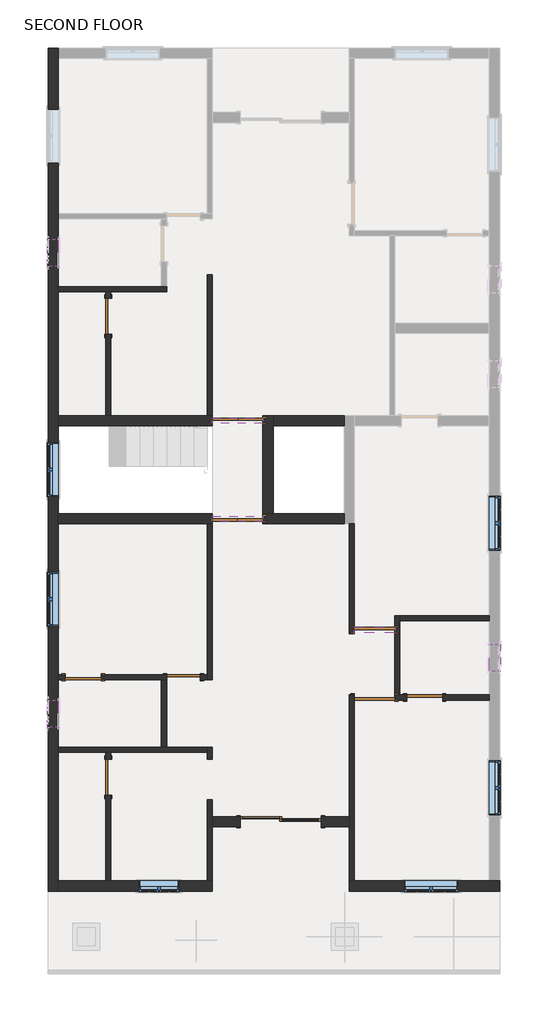
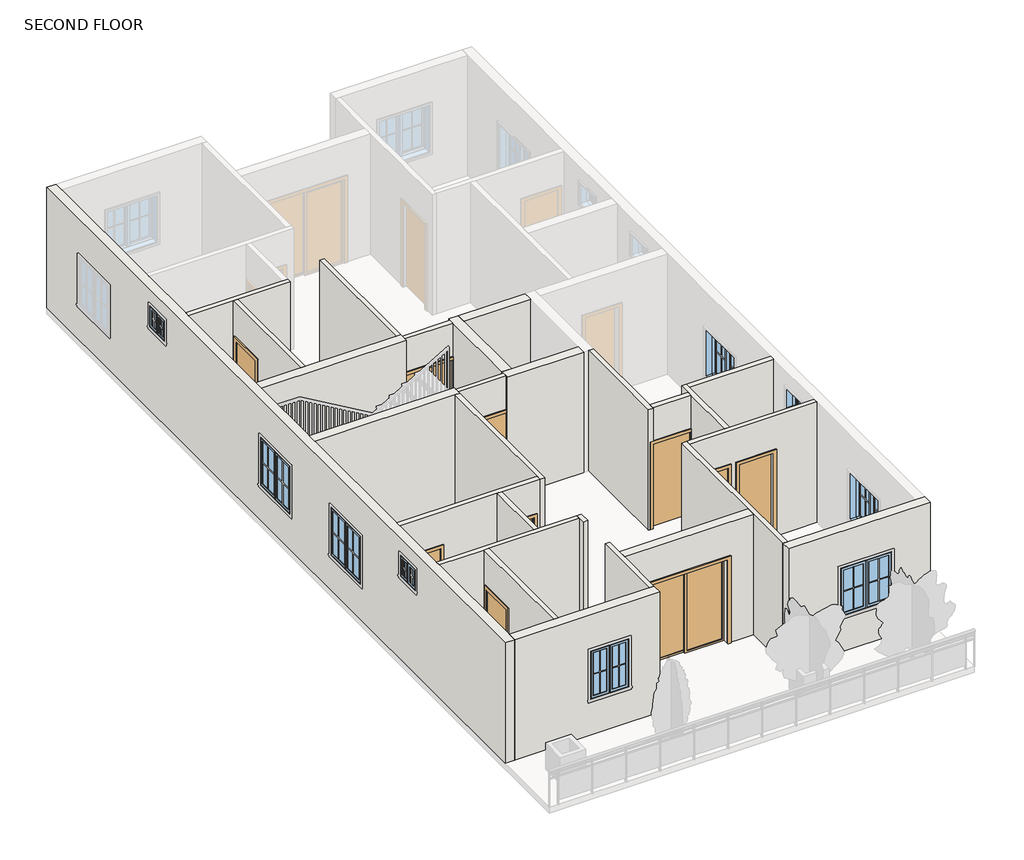
# One storey, part 1 of 4: 27 walls, 10 doors, 9 windows.
"""IFC4 building model written with IfcOpenShell, lengths in millimetres."""

from ifc_helpers import new_model, si_unit, frame, origin, place, context, project, spatial, polyline, outline, extrude, faceted_brep, transform, mapped, element, save
from components import door_31bd1cdd, door_d4d75d1e, door_214872d5, door_d141acb4, door_38851409, single_flush_3_x7_e5f9f3c4, single_flush_3_x7_305aa2a5, window_79894727, window_casement_double_3_x4_d341e8ac, window_casement_double_4_x4_af3140d2

model = new_model("IFC4")

# Units and contexts
model_context = context("Model", 3, world=origin())
ifc_project = project(units=[si_unit("LENGTHUNIT", "METRE", prefix="MILLI")], contexts=[model_context])

# Site, building, storey
site = spatial("IfcSite", under=ifc_project)
building = spatial("IfcBuilding", under=site)
storey = spatial("IfcBuildingStorey", under=building, Name="SECOND FLOOR", Elevation=6400.8)

# Doors
placement = place(None, origin())
door_shape = door_31bd1cdd(model_context)
element("IfcDoor", 1, ObjectType="Door-Double-Flush_Panel : 3'9\"X7'", at=placement, inside=storey, context=model_context, shape_type="MappedRepresentation", body=[
    mapped(door_shape, transform((-2091.0289041, 1664.1153263, 6400.8), x_axis=(1.0, 0.0, 0.0), y_axis=(0.0, 1.0, 0.0), z_axis=(0.0, 0.0, 1.0))),
])
element("IfcDoor", 2, ObjectType="Door-Double-Flush_Panel : 3'9\"X7'", at=placement, inside=storey, context=model_context, shape_type="MappedRepresentation", body=[
    mapped(door_shape, transform((-2091.0289041, -545.7007836, 6400.8), x_axis=(-1.0, 0.0, 0.0), y_axis=(0.0, -1.0, 0.0), z_axis=(0.0, 0.0, 1.0))),
])
door_2_shape = door_d4d75d1e(model_context)
element("IfcDoor", 3, ObjectType="Door-Double-Sliding : 72\" x 84\"", at=placement, inside=storey, context=model_context, shape_type="MappedRepresentation", body=[
    mapped(door_2_shape, transform((-1119.4789041, -7505.2846737, 6400.8), x_axis=(1.0, 0.0, 0.0), y_axis=(0.0, 1.0, 0.0), z_axis=(0.0, 0.0, 1.0))),
])
door_3_shape = door_214872d5(model_context)
element("IfcDoor", 4, ObjectType="Single-Flush : 2'6\"X7'", at=placement, inside=storey, context=model_context, shape_type="MappedRepresentation", body=[
    mapped(door_3_shape, transform((-3310.2289041, -4120.7346737, 6400.8), x_axis=(1.0, 0.0, 0.0), y_axis=(0.0, 1.0, 0.0), z_axis=(0.0, 0.0, 1.0))),
])
door_4_shape = door_d141acb4(model_context)
element("IfcDoor", 5, ObjectType="Single-Flush : 2'8\"X7'", at=placement, inside=storey, context=model_context, shape_type="MappedRepresentation", body=[
    mapped(door_4_shape, transform((-5005.6789041, 4013.6153263, 6400.8), x_axis=(0.0, 1.0, 0.0), y_axis=(-1.0, 0.0, 0.0), z_axis=(0.0, 0.0, 1.0))),
])
element("IfcDoor", 6, ObjectType="Single-Flush : 2'8\"X7'", at=placement, inside=storey, context=model_context, shape_type="MappedRepresentation", body=[
    mapped(door_4_shape, transform((-5570.8289041, -4120.7346737, 6400.8), x_axis=(-1.0, 0.0, 0.0), y_axis=(0.0, -1.0, 0.0), z_axis=(0.0, 0.0, 1.0))),
])
element("IfcDoor", 7, ObjectType="Single-Flush : 2'8\"X7'", at=placement, inside=storey, context=model_context, shape_type="MappedRepresentation", body=[
    mapped(door_4_shape, transform((-5005.6789041, -6374.9846737, 6400.8), x_axis=(0.0, 1.0, 0.0), y_axis=(-1.0, 0.0, 0.0), z_axis=(0.0, 0.0, 1.0))),
])
door_5_shape = door_38851409(model_context)
element("IfcDoor", 8, ObjectType="Single-Flush : 2'8\"X7'", at=placement, inside=storey, context=model_context, shape_type="MappedRepresentation", body=[
    mapped(door_5_shape, transform((2125.3710959, -4577.9346737, 6400.8), x_axis=(-1.0, 0.0, 0.0), y_axis=(0.0, -1.0, 0.0), z_axis=(0.0, 0.0, 1.0))),
])
single_flush_3_x7_shape = single_flush_3_x7_e5f9f3c4(model_context)
element("IfcDoor", 9, ObjectType="Single-Flush : 3'X7'", at=placement, inside=storey, context=model_context, shape_type="MappedRepresentation", body=[
    mapped(single_flush_3_x7_shape, transform((995.0710959, -4577.9346737, 6400.8), x_axis=(-1.0, 0.0, 0.0), y_axis=(0.0, -1.0, 0.0), z_axis=(0.0, 0.0, 1.0))),
])
single_flush_3_x7_2_shape = single_flush_3_x7_305aa2a5(model_context)
element("IfcDoor", 10, ObjectType="Single-Flush : 3'X7'", at=placement, inside=storey, context=model_context, shape_type="MappedRepresentation", body=[
    mapped(single_flush_3_x7_2_shape, transform((995.0710959, -3056.3085282, 6400.8), x_axis=(-1.0, 0.0, 0.0), y_axis=(0.0, -1.0, 0.0), z_axis=(0.0, 0.0, 1.0))),
])

# Walls
element("IfcWall", 11, ObjectType="4.5\"", at=placement, inside=storey, context=model_context, shape_type="Brep", body=[
    faceted_brep([(-6129.6289041, 4572.4153263, 6400.8), (-5062.8289041, 4572.4153263, 6400.8), (-4948.5289041, 4572.4153263, 6400.8), (-3691.2289041, 4572.4153263, 6400.8), (-3691.2289041, 4572.4153263, 9448.8), (-4948.5289041, 4572.4153263, 9448.8), (-5062.8289041, 4572.4153263, 9448.8), (-6129.6289041, 4572.4153263, 9448.8), (-6129.6289041, 4686.7153263, 6400.8), (-6129.6289041, 4686.7153263, 9448.8), (-3805.5289041, 4686.7153263, 9448.8), (-3691.2289041, 4686.7153263, 9448.8), (-3691.2289041, 4686.7153263, 6400.8), (-3805.5289041, 4686.7153263, 6400.8)], [[[0, 1, 2, 3, 4, 5, 6, 7]], [[8, 9, 10, 11, 12, 13]], [[3, 2, 1, 0, 8, 13, 12]], [[7, 6, 5, 4, 11, 10, 9]], [[0, 7, 9, 8]], [[4, 3, 12, 11]]]),
])
element("IfcWall", 12, ObjectType="4.5\"", at=placement, inside=storey, context=model_context, shape_type="SweptSolid", body=[
    extrude(outline(polyline([(4572.4153263, 6400.8), (4420.0153263, 6400.8), (4420.0153263, 8534.4), (3607.2153263, 8534.4), (3607.2153263, 6400.8), (1778.4153263, 6400.8), (1778.4153263, 9448.8), (4572.4153263, 9448.8), (4572.4153263, 6400.8)])), frame((-5062.8289041, 0.0, 0.0), z_axis=(1.0, 0.0, 0.0), x_axis=(0.0, 1.0, 0.0)), (0.0, 0.0, 1.0), 114.3),
])
element("IfcWall", 13, ObjectType="4.5\"", at=placement, inside=storey, context=model_context, shape_type="SweptSolid", body=[
    extrude(outline(polyline([(-2776.8289041, 1778.4153263), (-2776.8289041, 4948.2268555), (-2662.5289041, 4948.2268555), (-2662.5289041, 1778.4153263), (-2776.8289041, 1778.4153263)])), frame((0.0, 0.0, 6400.8), z_axis=(0.0, 0.0, 1.0), x_axis=(1.0, 0.0, 0.0)), (0.0, 0.0, 1.0), 3048.0),
])
element("IfcWall", 14, ObjectType="4.5\"", at=placement, inside=storey, context=model_context, shape_type="Brep", body=[
    faceted_brep([(-2776.8289041, -659.9846737, 6400.8), (-2776.8289041, -4063.5846737, 6400.8), (-2776.8289041, -4177.8846737, 6400.8), (-2776.8289041, -4177.8846737, 9448.8), (-2776.8289041, -4063.5846737, 9448.8), (-2776.8289041, -659.9846737, 9448.8), (-2662.5289041, -659.9846737, 6400.8), (-2662.5289041, -659.9846737, 9448.8), (-2662.5289041, -4177.8846737, 9448.8), (-2662.5289041, -4177.8846737, 6400.8)], [[[0, 1, 2, 3, 4, 5]], [[6, 7, 8, 9]], [[2, 1, 0, 6, 9]], [[5, 4, 3, 8, 7]], [[0, 5, 7, 6]], [[3, 2, 9, 8]]]),
])
element("IfcWall", 15, ObjectType="4.5\"", at=placement, inside=storey, context=model_context, shape_type="Brep", body=[
    faceted_brep([(-2776.8289041, -4063.5846737, 6400.8), (-2929.2289041, -4063.5846737, 6400.8), (-2929.2289041, -4063.5846737, 8534.4), (-3691.2289041, -4063.5846737, 8534.4), (-3691.2289041, -4063.5846737, 6400.8), (-5164.4289041, -4063.5846737, 6400.8), (-5164.4289041, -4063.5846737, 8534.4), (-5977.2289041, -4063.5846737, 8534.4), (-5977.2289041, -4063.5846737, 6400.8), (-6129.6289041, -4063.5846737, 6400.8), (-6129.6289041, -4063.5846737, 9448.8), (-2776.8289041, -4063.5846737, 9448.8), (-2929.2289041, -4177.8846737, 8534.4), (-2929.2289041, -4177.8846737, 6400.8), (-2776.8289041, -4177.8846737, 6400.8), (-2776.8289041, -4177.8846737, 9448.8), (-3691.2289041, -4177.8846737, 9448.8), (-3805.5289041, -4177.8846737, 9448.8), (-6129.6289041, -4177.8846737, 9448.8), (-6129.6289041, -4177.8846737, 6400.8), (-5977.2289041, -4177.8846737, 6400.8), (-5977.2289041, -4177.8846737, 8534.4), (-5164.4289041, -4177.8846737, 8534.4), (-5164.4289041, -4177.8846737, 6400.8), (-3805.5289041, -4177.8846737, 6400.8), (-3691.2289041, -4177.8846737, 6400.8), (-3691.2289041, -4177.8846737, 8534.4)], [[[0, 1, 2, 3, 4, 5, 6, 7, 8, 9, 10, 11]], [[12, 13, 14, 15, 16, 17, 18, 19, 20, 21, 22, 23, 24, 25, 26]], [[9, 8, 20, 19]], [[14, 13, 1, 0]], [[25, 24, 23, 5, 4]], [[11, 10, 18, 17, 16, 15]], [[0, 11, 15, 14]], [[10, 9, 19, 18]], [[21, 20, 8, 7]], [[22, 21, 7, 6]], [[23, 22, 6, 5]], [[2, 1, 13, 12]], [[3, 2, 12, 26]], [[4, 3, 26, 25]]]),
])
element("IfcWall", 16, ObjectType="4.5\"", at=placement, inside=storey, context=model_context, shape_type="Brep", body=[
    faceted_brep([(-3805.5289041, -4177.8846737, 6400.8), (-3805.5289041, -5701.8846737, 6400.8), (-3805.5289041, -5701.8846737, 9448.8), (-3805.5289041, -4177.8846737, 9448.8), (-3691.2289041, -4177.8846737, 6400.8), (-3691.2289041, -4177.8846737, 8534.4), (-3691.2289041, -4177.8846737, 9448.8), (-3691.2289041, -5701.8846737, 9448.8), (-3691.2289041, -5701.8846737, 6400.8)], [[[0, 1, 2, 3]], [[4, 5, 6, 7, 8]], [[1, 0, 4, 8]], [[3, 2, 7, 6]], [[0, 3, 6, 5, 4]], [[2, 1, 8, 7]]]),
])
element("IfcWall", 17, ObjectType="4.5\"", at=placement, inside=storey, context=model_context, shape_type="Brep", body=[
    faceted_brep([(-6129.6289041, -5816.1846737, 6400.8), (-5062.8289041, -5816.1846737, 6400.8), (-4948.5289041, -5816.1846737, 6400.8), (-2776.8289041, -5816.1846737, 6400.8), (-2776.8289041, -5816.1846737, 9448.8), (-4948.5289041, -5816.1846737, 9448.8), (-5062.8289041, -5816.1846737, 9448.8), (-6129.6289041, -5816.1846737, 9448.8), (-6129.6289041, -5701.8846737, 6400.8), (-6129.6289041, -5701.8846737, 9448.8), (-3805.5289041, -5701.8846737, 9448.8), (-3691.2289041, -5701.8846737, 9448.8), (-2776.8289041, -5701.8846737, 9448.8), (-2776.8289041, -5701.8846737, 6400.8), (-3691.2289041, -5701.8846737, 6400.8), (-3805.5289041, -5701.8846737, 6400.8)], [[[0, 1, 2, 3, 4, 5, 6, 7]], [[8, 9, 10, 11, 12, 13, 14, 15]], [[3, 2, 1, 0, 8, 15, 14, 13]], [[7, 6, 5, 4, 12, 11, 10, 9]], [[0, 7, 9, 8]], [[4, 3, 13, 12]]]),
])
element("IfcWall", 18, ObjectType="4.5\"", at=placement, inside=storey, context=model_context, shape_type="Brep", body=[
    faceted_brep([(-2776.8289041, -5701.8846737, 6400.8), (-2776.8289041, -5816.1846737, 6400.8), (-2776.8289041, -5968.5846737, 6400.8), (-2776.8289041, -5968.5846737, 9448.8), (-2776.8289041, -5816.1846737, 9448.8), (-2776.8289041, -5701.8846737, 9448.8), (-2662.5289041, -5701.8846737, 6400.8), (-2662.5289041, -5701.8846737, 9448.8), (-2662.5289041, -5968.5846737, 9448.8), (-2662.5289041, -5968.5846737, 6400.8)], [[[0, 1, 2, 3, 4, 5]], [[6, 7, 8, 9]], [[2, 1, 0, 6, 9]], [[3, 2, 9, 8]], [[5, 4, 3, 8, 7]], [[0, 5, 7, 6]]]),
])
element("IfcWall", 19, ObjectType="4.5\"", at=placement, inside=storey, context=model_context, shape_type="SweptSolid", body=[
    extrude(outline(polyline([(-5816.1846737, 6400.8), (-5968.5846737, 6400.8), (-5968.5846737, 8534.4), (-6781.3846737, 8534.4), (-6781.3846737, 6400.8), (-8711.7846737, 6400.8), (-8711.7846737, 9448.8), (-5816.1846737, 9448.8), (-5816.1846737, 6400.8)])), frame((-5062.8289041, 0.0, 0.0), z_axis=(1.0, 0.0, 0.0), x_axis=(0.0, 1.0, 0.0)), (0.0, 0.0, 1.0), 114.3),
])
element("IfcWall", 20, ObjectType="4.5\"", at=placement, inside=storey, context=model_context, shape_type="Brep", body=[
    faceted_brep([(-2776.8289041, -6882.9846737, 6400.8), (-2776.8289041, -8711.7846737, 6400.8), (-2776.8289041, -8711.7846737, 9448.8), (-2776.8289041, -6882.9846737, 9448.8), (-2662.5289041, -6882.9846737, 6400.8), (-2662.5289041, -6882.9846737, 9448.8), (-2662.5289041, -7263.9846737, 9448.8), (-2662.5289041, -7492.5846737, 9448.8), (-2662.5289041, -8711.7846737, 9448.8), (-2662.5289041, -8711.7846737, 6400.8), (-2662.5289041, -7492.5846737, 6400.8), (-2662.5289041, -7263.9846737, 6400.8)], [[[0, 1, 2, 3]], [[4, 5, 6, 7, 8, 9, 10, 11]], [[1, 0, 4, 11, 10, 9]], [[3, 2, 8, 7, 6, 5]], [[0, 3, 5, 4]], [[2, 1, 9, 8]]]),
])
element("IfcWall", 21, ObjectType="4.5\"", at=placement, inside=storey, context=model_context, shape_type="Brep", body=[
    faceted_brep([(423.5710959, -659.9846737, 6400.8), (423.5710959, -3136.3185282, 6400.8), (423.5710959, -3136.3185282, 9448.8), (423.5710959, -659.9846737, 9448.8), (537.8710959, -659.9846737, 6400.8), (537.8710959, -659.9846737, 9448.8), (537.8710959, -2999.1585282, 9448.8), (537.8710959, -3113.4585282, 9448.8), (537.8710959, -3136.3185282, 9448.8), (537.8710959, -3136.3185282, 6400.8), (537.8710959, -3113.4585282, 6400.8), (537.8710959, -2999.1585282, 6400.8)], [[[0, 1, 2, 3]], [[4, 5, 6, 7, 8, 9, 10, 11]], [[1, 0, 4, 11, 10, 9]], [[2, 1, 9, 8]], [[3, 2, 8, 7, 6, 5]], [[0, 3, 5, 4]]]),
])
element("IfcWall", 22, ObjectType="4.5\"", at=placement, inside=storey, context=model_context, shape_type="Brep", body=[
    faceted_brep([(423.5710959, -4520.7846737, 6400.8), (423.5710959, -7263.9846737, 6400.8), (423.5710959, -7492.5846737, 6400.8), (423.5710959, -8711.7846737, 6400.8), (423.5710959, -8711.7846737, 9448.8), (423.5710959, -7492.5846737, 9448.8), (423.5710959, -7263.9846737, 9448.8), (423.5710959, -4520.7846737, 9448.8), (537.8710959, -4520.7846737, 6400.8), (537.8710959, -4520.7846737, 8534.4), (537.8710959, -4520.7846737, 9448.8), (537.8710959, -4635.0846737, 9448.8), (537.8710959, -8711.7846737, 9448.8), (537.8710959, -8711.7846737, 6400.8)], [[[0, 1, 2, 3, 4, 5, 6, 7]], [[8, 9, 10, 11, 12, 13]], [[3, 2, 1, 0, 8, 13]], [[7, 6, 5, 4, 12, 11, 10]], [[4, 3, 13, 12]], [[0, 7, 10, 9, 8]]]),
])
element("IfcWall", 23, ObjectType="4.5\"", at=placement, inside=storey, context=model_context, shape_type="Brep", body=[
    faceted_brep([(1718.9710959, -4520.7846737, 8534.4), (1718.9710959, -4520.7846737, 6400.8), (1566.5710959, -4520.7846737, 6400.8), (1452.2710959, -4520.7846737, 6400.8), (1452.2710959, -4520.7846737, 8534.4), (537.8710959, -4520.7846737, 8534.4), (537.8710959, -4520.7846737, 9448.8), (1452.2710959, -4520.7846737, 9448.8), (1566.5710959, -4520.7846737, 9448.8), (3585.8710959, -4520.7846737, 9448.8), (3585.8710959, -4520.7846737, 6400.8), (2531.7710959, -4520.7846737, 6400.8), (2531.7710959, -4520.7846737, 8534.4), (1452.2710959, -4635.0846737, 6400.8), (1718.9710959, -4635.0846737, 6400.8), (1718.9710959, -4635.0846737, 8534.4), (2531.7710959, -4635.0846737, 8534.4), (2531.7710959, -4635.0846737, 6400.8), (3585.8710959, -4635.0846737, 6400.8), (3585.8710959, -4635.0846737, 9448.8), (537.8710959, -4635.0846737, 9448.8), (537.8710959, -4635.0846737, 8534.4), (1452.2710959, -4635.0846737, 8534.4)], [[[0, 1, 2, 3, 4, 5, 6, 7, 8, 9, 10, 11, 12]], [[13, 14, 15, 16, 17, 18, 19, 20, 21, 22]], [[11, 10, 18, 17]], [[3, 2, 1, 14, 13]], [[9, 8, 7, 6, 20, 19]], [[10, 9, 19, 18]], [[20, 6, 5, 21]], [[4, 22, 21, 5]], [[22, 4, 3, 13]], [[15, 14, 1, 0]], [[16, 15, 0, 12]], [[17, 16, 12, 11]]]),
])
element("IfcWall", 24, ObjectType="4.5\"", at=placement, inside=storey, context=model_context, shape_type="Brep", body=[
    faceted_brep([(1566.5710959, -4520.7846737, 6400.8), (1566.5710959, -2844.3846737, 6400.8), (1566.5710959, -2730.0846737, 6400.8), (1566.5710959, -2730.0846737, 9448.8), (1566.5710959, -2844.3846737, 9448.8), (1566.5710959, -4520.7846737, 9448.8), (1452.2710959, -4520.7846737, 6400.8), (1452.2710959, -4520.7846737, 8534.4), (1452.2710959, -4520.7846737, 9448.8), (1452.2710959, -3113.4585282, 9448.8), (1452.2710959, -2999.1585282, 9448.8), (1452.2710959, -2730.0846737, 9448.8), (1452.2710959, -2730.0846737, 6400.8), (1452.2710959, -2999.1585282, 6400.8), (1452.2710959, -3113.4585282, 6400.8)], [[[0, 1, 2, 3, 4, 5]], [[6, 7, 8, 9, 10, 11, 12, 13, 14]], [[2, 1, 0, 6, 14, 13, 12]], [[5, 4, 3, 11, 10, 9, 8]], [[0, 5, 8, 7, 6]], [[3, 2, 12, 11]]]),
])
element("IfcWall", 25, ObjectType="4.5\"", at=placement, inside=storey, context=model_context, shape_type="SweptSolid", body=[
    extrude(outline(polyline([(3585.8710959, -2844.3846737), (1566.5710959, -2844.3846737), (1566.5710959, -2730.0846737), (3585.8710959, -2730.0846737), (3585.8710959, -2844.3846737)])), frame((0.0, 0.0, 6400.8), z_axis=(0.0, 0.0, 1.0), x_axis=(1.0, 0.0, 0.0)), (0.0, 0.0, 1.0), 3048.0),
])
element("IfcWall", 26, ObjectType="4.5\"", at=placement, inside=storey, context=model_context, shape_type="SweptSolid", body=[
    extrude(outline(polyline([(-1519.5289041, 1606.9653263), (-2662.5289041, 1606.9653263), (-2662.5289041, 1721.2653263), (-1519.5289041, 1721.2653263), (-1519.5289041, 1606.9653263)])), frame((0.0, 0.0, 8534.4), z_axis=(0.0, 0.0, 1.0), x_axis=(1.0, 0.0, 0.0)), (0.0, 0.0, 1.0), 914.4),
])
element("IfcWall", 27, ObjectType="4.5\"", at=placement, inside=storey, context=model_context, shape_type="SweptSolid", body=[
    extrude(outline(polyline([(-1519.5289041, -602.8507836), (-2662.5289041, -602.8507836), (-2662.5289041, -488.5507836), (-1519.5289041, -488.5507836), (-1519.5289041, -602.8507836)])), frame((0.0, 0.0, 8534.4), z_axis=(0.0, 0.0, 1.0), x_axis=(1.0, 0.0, 0.0)), (0.0, 0.0, 1.0), 914.4),
])
element("IfcWall", 28, ObjectType="4.5\"", at=placement, inside=storey, context=model_context, shape_type="SweptSolid", body=[
    extrude(outline(polyline([(1452.2710959, -3113.4585282), (537.8710959, -3113.4585282), (537.8710959, -2999.1585282), (1452.2710959, -2999.1585282), (1452.2710959, -3113.4585282)])), frame((0.0, 0.0, 8534.4), z_axis=(0.0, 0.0, 1.0), x_axis=(1.0, 0.0, 0.0)), (0.0, 0.0, 1.0), 914.4),
])
element("IfcWall", 29, ObjectType="9\"", at=placement, inside=storey, context=model_context, shape_type="Brep", body=[
    faceted_brep([(-6358.2289041, 10058.8153263, 6400.8), (-6358.2289041, -8940.3846737, 6400.8), (-6358.2289041, -8940.3846737, 9448.8), (-6358.2289041, 10058.8153263, 9448.8), (-6358.2289041, 8687.2153263, 8534.4), (-6358.2289041, 7468.0153263, 8534.4), (-6358.2289041, 7468.0153263, 7315.2), (-6358.2289041, 8687.2153263, 7315.2), (-6358.2289041, -1752.1846737, 8534.4), (-6358.2289041, -2971.3846737, 8534.4), (-6358.2289041, -2971.3846737, 7315.2), (-6358.2289041, -1752.1846737, 7315.2), (-6358.2289041, 1168.8153263, 8534.4), (-6358.2289041, -50.3846737, 8534.4), (-6358.2289041, -50.3846737, 7315.2), (-6358.2289041, 1168.8153263, 7315.2), (-6358.2289041, 5753.5153263, 9067.8), (-6358.2289041, 5143.9153263, 9067.8), (-6358.2289041, 5143.9153263, 8534.4), (-6358.2289041, 5753.5153263, 8534.4), (-6358.2289041, -4635.0846737, 9067.8), (-6358.2289041, -5244.6846737, 9067.8), (-6358.2289041, -5244.6846737, 8534.4), (-6358.2289041, -4635.0846737, 8534.4), (-6129.6289041, 10058.8153263, 6400.8), (-6129.6289041, 10058.8153263, 9448.8), (-6129.6289041, 9830.2153263, 9448.8), (-6129.6289041, 6325.0153263, 9448.8), (-6129.6289041, 6210.7153263, 9448.8), (-6129.6289041, 4686.7153263, 9448.8), (-6129.6289041, 4572.4153263, 9448.8), (-6129.6289041, 1778.4153263, 9448.8), (-6129.6289041, 1549.8153263, 9448.8), (-6129.6289041, -431.3846737, 9448.8), (-6129.6289041, -659.9846737, 9448.8), (-6129.6289041, -4063.5846737, 9448.8), (-6129.6289041, -4177.8846737, 9448.8), (-6129.6289041, -5701.8846737, 9448.8), (-6129.6289041, -5816.1846737, 9448.8), (-6129.6289041, -8711.7846737, 9448.8), (-6129.6289041, -8940.3846737, 9448.8), (-6129.6289041, -8940.3846737, 6400.8), (-6129.6289041, -8711.7846737, 6400.8), (-6129.6289041, -5816.1846737, 6400.8), (-6129.6289041, -5701.8846737, 6400.8), (-6129.6289041, -4177.8846737, 6400.8), (-6129.6289041, -4063.5846737, 6400.8), (-6129.6289041, -659.9846737, 6400.8), (-6129.6289041, -431.3846737, 6400.8), (-6129.6289041, 1549.8153263, 6400.8), (-6129.6289041, 1778.4153263, 6400.8), (-6129.6289041, 4572.4153263, 6400.8), (-6129.6289041, 4686.7153263, 6400.8), (-6129.6289041, 6210.7153263, 6400.8), (-6129.6289041, 6325.0153263, 6400.8), (-6129.6289041, 9830.2153263, 6400.8), (-6129.6289041, 8687.2153263, 8534.4), (-6129.6289041, 8687.2153263, 7315.2), (-6129.6289041, 7468.0153263, 7315.2), (-6129.6289041, 7468.0153263, 8534.4), (-6129.6289041, -1752.1846737, 8534.4), (-6129.6289041, -1752.1846737, 7315.2), (-6129.6289041, -2971.3846737, 7315.2), (-6129.6289041, -2971.3846737, 8534.4), (-6129.6289041, 1168.8153263, 8534.4), (-6129.6289041, 1168.8153263, 7315.2), (-6129.6289041, -50.3846737, 7315.2), (-6129.6289041, -50.3846737, 8534.4), (-6129.6289041, 5753.5153263, 9067.8), (-6129.6289041, 5753.5153263, 8534.4), (-6129.6289041, 5143.9153263, 8534.4), (-6129.6289041, 5143.9153263, 9067.8), (-6129.6289041, -4635.0846737, 9067.8), (-6129.6289041, -4635.0846737, 8534.4), (-6129.6289041, -5244.6846737, 8534.4), (-6129.6289041, -5244.6846737, 9067.8)], [[[0, 1, 2, 3], [4, 5, 6, 7], [8, 9, 10, 11], [12, 13, 14, 15], [16, 17, 18, 19], [20, 21, 22, 23]], [[24, 25, 26, 27, 28, 29, 30, 31, 32, 33, 34, 35, 36, 37, 38, 39, 40, 41, 42, 43, 44, 45, 46, 47, 48, 49, 50, 51, 52, 53, 54, 55], [56, 57, 58, 59], [60, 61, 62, 63], [64, 65, 66, 67], [68, 69, 70, 71], [72, 73, 74, 75]], [[1, 0, 24, 55, 54, 53, 52, 51, 50, 49, 48, 47, 46, 45, 44, 43, 42, 41]], [[3, 2, 40, 39, 38, 37, 36, 35, 34, 33, 32, 31, 30, 29, 28, 27, 26, 25]], [[2, 1, 41, 40]], [[0, 3, 25, 24]], [[57, 56, 4, 7]], [[58, 57, 7, 6]], [[59, 58, 6, 5]], [[56, 59, 5, 4]], [[61, 60, 8, 11]], [[62, 61, 11, 10]], [[63, 62, 10, 9]], [[60, 63, 9, 8]], [[65, 64, 12, 15]], [[66, 65, 15, 14]], [[67, 66, 14, 13]], [[64, 67, 13, 12]], [[69, 68, 16, 19]], [[70, 69, 19, 18]], [[71, 70, 18, 17]], [[68, 71, 17, 16]], [[73, 72, 20, 23]], [[74, 73, 23, 22]], [[75, 74, 22, 21]], [[72, 75, 21, 20]]]),
])
element("IfcWall", 30, ObjectType="9\"", at=placement, inside=storey, context=model_context, shape_type="Brep", body=[
    faceted_brep([(-6129.6289041, -8940.3846737, 6400.8), (-2662.5289041, -8940.3846737, 6400.8), (-2662.5289041, -8940.3846737, 9448.8), (-6129.6289041, -8940.3846737, 9448.8), (-4319.8789041, -8940.3846737, 8534.4), (-3405.4789041, -8940.3846737, 8534.4), (-3405.4789041, -8940.3846737, 7315.2), (-4319.8789041, -8940.3846737, 7315.2), (-6129.6289041, -8711.7846737, 6400.8), (-6129.6289041, -8711.7846737, 9448.8), (-5062.8289041, -8711.7846737, 9448.8), (-4948.5289041, -8711.7846737, 9448.8), (-2776.8289041, -8711.7846737, 9448.8), (-2662.5289041, -8711.7846737, 9448.8), (-2662.5289041, -8711.7846737, 6400.8), (-2776.8289041, -8711.7846737, 6400.8), (-4948.5289041, -8711.7846737, 6400.8), (-5062.8289041, -8711.7846737, 6400.8), (-4319.8789041, -8711.7846737, 8534.4), (-4319.8789041, -8711.7846737, 7315.2), (-3405.4789041, -8711.7846737, 7315.2), (-3405.4789041, -8711.7846737, 8534.4)], [[[0, 1, 2, 3], [4, 5, 6, 7]], [[8, 9, 10, 11, 12, 13, 14, 15, 16, 17], [18, 19, 20, 21]], [[1, 0, 8, 17, 16, 15, 14]], [[3, 2, 13, 12, 11, 10, 9]], [[0, 3, 9, 8]], [[2, 1, 14, 13]], [[19, 18, 4, 7]], [[20, 19, 7, 6]], [[21, 20, 6, 5]], [[18, 21, 5, 4]]]),
])
element("IfcWall", 31, ObjectType="9\"", at=placement, inside=storey, context=model_context, shape_type="Brep", body=[
    faceted_brep([(423.5710959, -8940.3846737, 6400.8), (3814.4710959, -8940.3846737, 6400.8), (3814.4710959, -8940.3846737, 9448.8), (423.5710959, -8940.3846737, 9448.8), (1662.2107801, -8940.3846737, 8534.4), (2881.4107801, -8940.3846737, 8534.4), (2881.4107801, -8940.3846737, 7315.2), (1662.2107801, -8940.3846737, 7315.2), (423.5710959, -8711.7846737, 6400.8), (423.5710959, -8711.7846737, 9448.8), (537.8710959, -8711.7846737, 9448.8), (3585.8710959, -8711.7846737, 9448.8), (3814.4710959, -8711.7846737, 9448.8), (3814.4710959, -8711.7846737, 6400.8), (3585.8710959, -8711.7846737, 6400.8), (537.8710959, -8711.7846737, 6400.8), (1662.2107801, -8711.7846737, 8534.4), (1662.2107801, -8711.7846737, 7315.2), (2881.4107801, -8711.7846737, 7315.2), (2881.4107801, -8711.7846737, 8534.4)], [[[0, 1, 2, 3], [4, 5, 6, 7]], [[8, 9, 10, 11, 12, 13, 14, 15], [16, 17, 18, 19]], [[1, 0, 8, 15, 14, 13]], [[3, 2, 12, 11, 10, 9]], [[2, 1, 13, 12]], [[0, 3, 9, 8]], [[17, 16, 4, 7]], [[18, 17, 7, 6]], [[19, 18, 6, 5]], [[16, 19, 5, 4]]]),
])
element("IfcWall", 32, ObjectType="9\"", at=placement, inside=storey, context=model_context, shape_type="Brep", body=[
    faceted_brep([(-6129.6289041, 1549.8153263, 6400.8), (-2662.5289041, 1549.8153263, 6400.8), (-2662.5289041, 1549.8153263, 9448.8), (-6129.6289041, 1549.8153263, 9448.8), (-6129.6289041, 1778.4153263, 6400.8), (-6129.6289041, 1778.4153263, 9448.8), (-5062.8289041, 1778.4153263, 9448.8), (-4948.5289041, 1778.4153263, 9448.8), (-2776.8289041, 1778.4153263, 9448.8), (-2662.5289041, 1778.4153263, 9448.8), (-2662.5289041, 1778.4153263, 6400.8), (-2776.8289041, 1778.4153263, 6400.8), (-4948.5289041, 1778.4153263, 6400.8), (-5062.8289041, 1778.4153263, 6400.8), (-2662.5289041, 1606.9653263, 9448.8), (-2662.5289041, 1721.2653263, 9448.8)], [[[0, 1, 2, 3]], [[4, 5, 6, 7, 8, 9, 10, 11, 12, 13]], [[1, 0, 4, 13, 12, 11, 10]], [[3, 2, 14, 15, 9, 8, 7, 6, 5]], [[0, 3, 5, 4]], [[2, 1, 10, 9, 15, 14]]]),
])
element("IfcWall", 33, ObjectType="9\"", at=placement, inside=storey, context=model_context, shape_type="Brep", body=[
    faceted_brep([(-6129.6289041, -659.9846737, 6400.8), (-2776.8289041, -659.9846737, 6400.8), (-2662.5289041, -659.9846737, 6400.8), (-2662.5289041, -659.9846737, 9448.8), (-2776.8289041, -659.9846737, 9448.8), (-6129.6289041, -659.9846737, 9448.8), (-6129.6289041, -431.3846737, 6400.8), (-6129.6289041, -431.3846737, 9448.8), (-2662.5289041, -431.3846737, 9448.8), (-2662.5289041, -431.3846737, 6400.8), (-2662.5289041, -602.8507836, 9448.8), (-2662.5289041, -488.5507836, 9448.8)], [[[0, 1, 2, 3, 4, 5]], [[6, 7, 8, 9]], [[2, 1, 0, 6, 9]], [[5, 4, 3, 10, 11, 8, 7]], [[0, 5, 7, 6]], [[3, 2, 9, 8, 11, 10]]]),
])
element("IfcWall", 34, ObjectType="9\"", at=placement, inside=storey, context=model_context, shape_type="Brep", body=[
    faceted_brep([(309.2710959, -431.3846737, 6400.8), (-1290.9289041, -431.3846737, 6400.8), (-1519.5289041, -431.3846737, 6400.8), (-1519.5289041, -431.3846737, 9448.8), (-1290.9289041, -431.3846737, 9448.8), (309.2710959, -431.3846737, 9448.8), (309.2710959, -659.9846737, 6400.8), (309.2710959, -659.9846737, 9448.8), (-1519.5289041, -659.9846737, 9448.8), (-1519.5289041, -659.9846737, 6400.8), (-1519.5289041, -488.5507836, 9448.8), (-1519.5289041, -602.8507836, 9448.8)], [[[0, 1, 2, 3, 4, 5]], [[6, 7, 8, 9]], [[2, 1, 0, 6, 9]], [[5, 4, 3, 10, 11, 8, 7]], [[0, 5, 7, 6]], [[3, 2, 9, 8, 11, 10]]]),
])
element("IfcWall", 35, ObjectType="9\"", at=placement, inside=storey, context=model_context, shape_type="Brep", body=[
    faceted_brep([(-1290.9289041, -431.3846737, 6400.8), (-1290.9289041, 1549.8153263, 6400.8), (-1290.9289041, 1778.4153263, 6400.8), (-1290.9289041, 1778.4153263, 9448.8), (-1290.9289041, 1549.8153263, 9448.8), (-1290.9289041, -431.3846737, 9448.8), (-1519.5289041, -431.3846737, 6400.8), (-1519.5289041, -431.3846737, 9448.8), (-1519.5289041, 1606.9653263, 9448.8), (-1519.5289041, 1721.2653263, 9448.8), (-1519.5289041, 1778.4153263, 9448.8), (-1519.5289041, 1778.4153263, 6400.8)], [[[0, 1, 2, 3, 4, 5]], [[6, 7, 8, 9, 10, 11]], [[2, 1, 0, 6, 11]], [[5, 4, 3, 10, 9, 8, 7]], [[0, 5, 7, 6]], [[3, 2, 11, 10]]]),
])
element("IfcWall", 36, ObjectType="9\"", at=placement, inside=storey, context=model_context, shape_type="SweptSolid", body=[
    extrude(outline(polyline([(-1290.9289041, 1778.4153263), (309.2710959, 1778.4153263), (309.2710959, 1549.8153263), (-1290.9289041, 1549.8153263), (-1290.9289041, 1778.4153263)])), frame((0.0, 0.0, 6400.8), z_axis=(0.0, 0.0, 1.0), x_axis=(1.0, 0.0, 0.0)), (0.0, 0.0, 1.0), 3048.0),
])
element("IfcWall", 37, ObjectType="9\"", at=placement, inside=storey, context=model_context, shape_type="SweptSolid", body=[
    extrude(outline(polyline([(8534.4, -205.0789041), (6400.8, -205.0789041), (6400.8, 423.5710959), (9448.8, 423.5710959), (9448.8, -2662.5289041), (6400.8, -2662.5289041), (6400.8, -2033.8789041), (8534.4, -2033.8789041), (8534.4, -205.0789041)])), frame((0.0, -7492.5846737, 0.0), z_axis=(0.0, 1.0, 0.0), x_axis=(0.0, 0.0, 1.0)), (0.0, 0.0, 1.0), 228.6),
])

# Windows
window_shape = window_79894727(model_context)
element("IfcWindow", 38, ObjectType="Window-Casement-Double : 2'X1'9\"", at=placement, inside=storey, context=model_context, shape_type="MappedRepresentation", body=[
    mapped(window_shape, transform((-6243.9289041, 5448.7153263, 6400.8), x_axis=(0.0, 1.0, 0.0), y_axis=(-1.0, 0.0, 0.0), z_axis=(0.0, 0.0, 1.0))),
])
element("IfcWindow", 39, ObjectType="Window-Casement-Double : 2'X1'9\"", at=placement, inside=storey, context=model_context, shape_type="MappedRepresentation", body=[
    mapped(window_shape, transform((-6243.9289041, -4939.8846737, 6400.8), x_axis=(0.0, 1.0, 0.0), y_axis=(-1.0, 0.0, 0.0), z_axis=(0.0, 0.0, 1.0))),
])
element("IfcWindow", 40, ObjectType="Window-Casement-Double : 2'X1'9\"", at=placement, inside=storey, context=model_context, shape_type="MappedRepresentation", body=[
    mapped(window_shape, transform((3700.1710959, -3682.5846737, 6400.8), x_axis=(0.0, -1.0, 0.0), y_axis=(1.0, 0.0, 0.0), z_axis=(0.0, 0.0, 1.0))),
])
window_casement_double_3_x4_shape = window_casement_double_3_x4_d341e8ac(model_context)
element("IfcWindow", 41, ObjectType="Window-Casement-Double : 3'X4'", at=placement, inside=storey, context=model_context, shape_type="MappedRepresentation", body=[
    mapped(window_casement_double_3_x4_shape, transform((-3862.6789041, -8826.0846737, 6400.8), x_axis=(-1.0, 0.0, 0.0), y_axis=(0.0, -1.0, 0.0), z_axis=(0.0, 0.0, 1.0))),
])
window_casement_double_4_x4_shape = window_casement_double_4_x4_af3140d2(model_context)
element("IfcWindow", 42, ObjectType="Window-Casement-Double : 4'X4'", at=placement, inside=storey, context=model_context, shape_type="MappedRepresentation", body=[
    mapped(window_casement_double_4_x4_shape, transform((-6243.9289041, -2361.7846737, 6400.8), x_axis=(0.0, 1.0, 0.0), y_axis=(-1.0, 0.0, 0.0), z_axis=(0.0, 0.0, 1.0))),
])
element("IfcWindow", 43, ObjectType="Window-Casement-Double : 4'X4'", at=placement, inside=storey, context=model_context, shape_type="MappedRepresentation", body=[
    mapped(window_casement_double_4_x4_shape, transform((2271.8107801, -8826.0846737, 6400.8), x_axis=(-1.0, 0.0, 0.0), y_axis=(0.0, -1.0, 0.0), z_axis=(0.0, 0.0, 1.0))),
])
element("IfcWindow", 44, ObjectType="Window-Casement-Double : 4'X4'", at=placement, inside=storey, context=model_context, shape_type="MappedRepresentation", body=[
    mapped(window_casement_double_4_x4_shape, transform((3700.1710959, -6616.2846737, 6400.8), x_axis=(0.0, -1.0, 0.0), y_axis=(1.0, 0.0, 0.0), z_axis=(0.0, 0.0, 1.0))),
])
element("IfcWindow", 45, ObjectType="Window-Casement-Double : 4'X4'", at=placement, inside=storey, context=model_context, shape_type="MappedRepresentation", body=[
    mapped(window_casement_double_4_x4_shape, transform((3700.1710959, -647.2846737, 6400.8), x_axis=(0.0, -1.0, 0.0), y_axis=(1.0, 0.0, 0.0), z_axis=(0.0, 0.0, 1.0))),
])
element("IfcWindow", 46, ObjectType="Window-Casement-Double : 4'X4'", at=placement, inside=storey, context=model_context, shape_type="MappedRepresentation", body=[
    mapped(window_casement_double_4_x4_shape, transform((-6243.9289041, 559.2153263, 6400.8), x_axis=(0.0, 1.0, 0.0), y_axis=(-1.0, 0.0, 0.0), z_axis=(0.0, 0.0, 1.0))),
])

save(model, "model.ifc")

# Revit data of these elements
# Type "Door-Double-Flush_Panel : 3'9\"X7'"
#   Type Mark = "11"
#   Construction Type Id = "DOOR"
#   Assembly Code = "C1020"
#   Analytic Construction = "Wooden"
#   Thickness = 0' - 2"
#   Thermal Resistance (R) = 2.5876 (h·ft²·°F)/BTU
#   Swing Angle [instance default] = 90.00°
#   Panel Width = 1' - 10 1/2"
#   Heat Transfer Coefficient (U) = 0.3865 BTU/(h·ft²·°F)
#   Height = 7' - 0"
#   Trim Projection Ext = 0' - 1"
#   Trim Projection Int = 0' - 1"
#   Trim Width = 0' - 3"
#   Width = 3' - 9"
#   Define Thermal Properties by = 1
#   Panel Material = Wood - Birch - Solid Stained Light Low Gloss
#   Trim Material = Paint - Sienna
#   Visual Light Transmittance = 0
#   Solar Heat Gain Coefficient = 0
#   Function = (empty or 0)
#   Wall Closure = (empty or 0)
# Type "Door-Double-Sliding : 72\" x 84\""
#   Type Mark = "14"
#   Construction Type Id = "opn-d45"
#   Assembly Code = "C1020"
#   Analytic Construction = "Wood frame, double glass door "
#   Thickness = 0' - 2"
#   Thermal Resistance (R) = 1.8150 (h·ft²·°F)/BTU
#   Heat Transfer Coefficient (U) = 0.5510 BTU/(h·ft²·°F)
#   Height = 7' - 0"
#   Rail Width = 0' - 2"
#   Stiles = 0' - 2"
#   Trim Projection Ext = 0' - 1"
#   Trim Projection Int = 0' - 1"
#   Trim Width = 0' - 3"
#   Width = 6' - 0"
#   Define Thermal Properties by = 1
#   Glazing = Glass
#   Panel Material = Wood - Birch - Solid Stained Light Low Gloss
#   Trim Material = Paint - Sienna
#   Visual Light Transmittance = 0
#   Solar Heat Gain Coefficient = 0
#   Function = (empty or 0)
#   Wall Closure = (empty or 0)
# Type "Single-Flush : 2'6\"X7'"
#   Type Mark = "13"
#   Construction Type Id = "MDOOR"
#   Assembly Code = "C1020"
#   Analytic Construction = "Metal"
#   Thickness = 0' - 2"
#   Heat Transfer Coefficient (U) = 0.651978 BTU/(h·ft²·°F)
#   Height = 7' - 0"
#   Trim Projection Ext = 0' - 1"
#   Trim Projection Int = 0' - 1"
#   Trim Width = 0' - 3"
#   Width = 2' - 6"
#   Define Thermal Properties by = 1
#   Door Material = Door - Panel
#   Frame Material = Door - Frame
#   Visual Light Transmittance = 0
#   Solar Heat Gain Coefficient = 0
#   Function = (empty or 0)
#   Wall Closure = (empty or 0)
# Type "Single-Flush : 2'8\"X7'"
#   Type Mark = "12"
#   Construction Type Id = "MDOOR"
#   Assembly Code = "C1020"
#   Analytic Construction = "Metal"
#   Thickness = 0' - 2"
#   Heat Transfer Coefficient (U) = 0.651978 BTU/(h·ft²·°F)
#   Height = 7' - 0"
#   Trim Projection Ext = 0' - 1"
#   Trim Projection Int = 0' - 1"
#   Trim Width = 0' - 3"
#   Width = 2' - 8"
#   Define Thermal Properties by = 1
#   Door Material = Door - Panel
#   Frame Material = Door - Frame
#   Visual Light Transmittance = 0
#   Solar Heat Gain Coefficient = 0
#   Function = (empty or 0)
#   Wall Closure = (empty or 0)
# Type "Single-Flush : 3'X7'"
#   Type Mark = "8"
#   Construction Type Id = "MDOOR"
#   Assembly Code = "C1020"
#   Analytic Construction = "Metal"
#   Thickness = 0' - 2"
#   Heat Transfer Coefficient (U) = 0.651978 BTU/(h·ft²·°F)
#   Height = 7' - 0"
#   Trim Projection Ext = 0' - 1"
#   Trim Projection Int = 0' - 1"
#   Trim Width = 0' - 3"
#   Width = 3' - 0"
#   Define Thermal Properties by = 1
#   Door Material = Door - Panel
#   Frame Material = Door - Frame
#   Visual Light Transmittance = 0
#   Solar Heat Gain Coefficient = 0
#   Function = (empty or 0)
#   Wall Closure = (empty or 0)
# Type "4.5\""
#   Assembly Code = "B2010"
#   Layers, outside or top first: 0' - 4 1/2" no material (function 1)
# Type "9\""
#   Assembly Code = "B2010"
#   Layers, outside or top first: 0' - 9" "WALL" (function 1)
# Type "Window-Casement-Double : 2'X1'9\""
#   Type Mark = "22"
#   Fire Rating = "0.5h"
#   Assembly Code = "B2020100"
#   Analytic Construction = "Double glazing - domestic"
#   Frame Extension [instance default] = 0' - 0 1/4"
#   Window Inset [instance default] = 0' - 0"
#   Wall Thickness [instance default] = 0' - 6"
#   Interior Wall Closure [instance default] = 0' - 2 1/4"
#   Half Width = 1' - 0"
#   Visual Light Transmittance = 0.81
#   Thermal Resistance (R) = 1.8146 (h·ft²·°F)/BTU
#   Solar Heat Gain Coefficient = 0.76
#   Rough Width = 2' - 0 1/2"
#   Rough Height = 1' - 9 1/2"
#   Height = 1' - 9"
#   Heat Transfer Coefficient (U) = 0.5511 BTU/(h·ft²·°F)
#   Exterior Wall Closure [instance default] = 0' - 1 1/4"
#   Extension Jamb [instance default] = 0' - 2 1/4"
#   Default Sill Height = 7' - 0"
#   Width = 2' - 0"
#   Muntin Visibility = yes
#   Interior Trim Visibility [instance default] = yes
#   Exterior Trim Visibility [instance default] = yes
#   Extension Jamb Visibility [instance default] = yes
#   Interior Trim Material = Wood - Stained
#   Muntin Pattern = Muntin Pattern_2x2 : Muntin Pattern_2x2
#   Interior Trim = Trim-Window-Interior-Flat : Picture Frame
#   Interior Frame Material = Wood - Stained
#   Glass Panel Material = Glass
#   Exterior Trim Material = Clad - White
#   Exterior Trim = Trim-Window-Exterior-Flat : with Sill
#   Exterior Frame Material = Clad - White
#   Wall Closure = (empty or 0)
# Type "Window-Casement-Double : 3'X4'"
#   Type Mark = "21"
#   Fire Rating = "0.5h"
#   Assembly Code = "B2020100"
#   Analytic Construction = "Double glazing - domestic"
#   Frame Extension [instance default] = 0' - 0 1/4"
#   Window Inset [instance default] = 0' - 0"
#   Wall Thickness [instance default] = 0' - 6"
#   Interior Wall Closure [instance default] = 0' - 2 1/4"
#   Half Width = 1' - 6"
#   Visual Light Transmittance = 0.81
#   Thermal Resistance (R) = 1.8146 (h·ft²·°F)/BTU
#   Solar Heat Gain Coefficient = 0.76
#   Rough Width = 3' - 0 1/2"
#   Rough Height = 4' - 0 1/2"
#   Height = 4' - 0"
#   Heat Transfer Coefficient (U) = 0.5511 BTU/(h·ft²·°F)
#   Exterior Wall Closure [instance default] = 0' - 1 1/4"
#   Extension Jamb [instance default] = 0' - 2 1/4"
#   Default Sill Height = 3' - 0"
#   Width = 3' - 0"
#   Muntin Visibility = yes
#   Interior Trim Visibility [instance default] = yes
#   Exterior Trim Visibility [instance default] = yes
#   Extension Jamb Visibility [instance default] = yes
#   Interior Trim Material = Wood - Stained
#   Muntin Pattern = Muntin Pattern_2x2 : Muntin Pattern_2x2
#   Interior Trim = Trim-Window-Interior-Flat : Picture Frame
#   Interior Frame Material = Wood - Stained
#   Glass Panel Material = Glass
#   Exterior Trim Material = Clad - White
#   Exterior Trim = Trim-Window-Exterior-Flat : with Sill
#   Exterior Frame Material = Clad - White
#   Wall Closure = (empty or 0)
# Type "Window-Casement-Double : 4'X4'"
#   Type Mark = "20"
#   Fire Rating = "0.5h"
#   Assembly Code = "B2020100"
#   Analytic Construction = "Double glazing - domestic"
#   Frame Extension [instance default] = 0' - 0 1/4"
#   Window Inset [instance default] = 0' - 0"
#   Wall Thickness [instance default] = 0' - 6"
#   Interior Wall Closure [instance default] = 0' - 2 1/4"
#   Half Width = 2' - 0"
#   Visual Light Transmittance = 0.81
#   Thermal Resistance (R) = 1.8146 (h·ft²·°F)/BTU
#   Solar Heat Gain Coefficient = 0.76
#   Rough Width = 4' - 0 1/2"
#   Rough Height = 4' - 0 1/2"
#   Height = 4' - 0"
#   Heat Transfer Coefficient (U) = 0.5511 BTU/(h·ft²·°F)
#   Exterior Wall Closure [instance default] = 0' - 1 1/4"
#   Extension Jamb [instance default] = 0' - 2 1/4"
#   Default Sill Height = 3' - 0"
#   Width = 4' - 0"
#   Muntin Visibility = yes
#   Interior Trim Visibility [instance default] = yes
#   Exterior Trim Visibility [instance default] = yes
#   Extension Jamb Visibility [instance default] = yes
#   Interior Trim Material = Wood - Stained
#   Muntin Pattern = Muntin Pattern_2x2 : Muntin Pattern_2x2
#   Interior Trim = Trim-Window-Interior-Flat : Picture Frame
#   Interior Frame Material = Wood - Stained
#   Glass Panel Material = Glass
#   Exterior Trim Material = Clad - White
#   Exterior Trim = Trim-Window-Exterior-Flat : with Sill
#   Exterior Frame Material = Clad - White
#   Wall Closure = (empty or 0)
# Elements 1, 2 (IfcDoor, "Door-Double-Flush_Panel : 3'9\"X7'")
#   Swing Angle = 90.00°
#   Phase Created = New Construction
#   Materials on its faces: "Paint - Sienna", "Wood - Birch - Solid Stained Light Low Gloss"
# Element 3 (IfcDoor, "Door-Double-Sliding : 72\" x 84\"")
#   Phase Created = New Construction
#   Materials on its faces: "Paint - Sienna", "Wood - Birch - Solid Stained Light Low Gloss", "Glass"
# Element 4 (IfcDoor, "Single-Flush : 2'6\"X7'")
#   Phase Created = New Construction
#   Materials on its faces: "Door - Frame", "Door - Panel"
# Elements 5, 6, 7, 8 (IfcDoor, "Single-Flush : 2'8\"X7'")
#   Phase Created = New Construction
#   Materials on its faces: "Door - Frame", "Door - Panel"
# Elements 9, 10 (IfcDoor, "Single-Flush : 3'X7'")
#   Phase Created = New Construction
#   Materials on its faces: "Door - Frame", "Door - Panel"
# Elements 11, 12, 13, 14, 15, 16, 17, 18, 19, 20, 21, 22, 23, 24, 25, 26, 27, 28 (IfcWall, "4.5\"")
#   Top Offset = -0' - 6"
#   Base Offset = 0' - 0"
#   wall height = 10' - 0"
#   Phase Created = New Construction
#   Base Constraint = SECOND FLOOR
#   Top Constraint = THIRD FLOOR
#   Materials on its faces: "Default Wall"
# Element 29 (IfcWall, "9\"")
#   Top Offset = -0' - 6"
#   Base Offset = 0' - 0"
#   wall height = 10' - 0"
#   Phase Created = New Construction
#   Base Constraint = SECOND FLOOR
#   Top Constraint = THIRD FLOOR
#   Materials on its faces: "WALL", "6\" WALL"
# Elements 30, 32, 33 (IfcWall, "9\"")
#   Top Offset = -0' - 6"
#   Base Offset = 0' - 0"
#   wall height = 10' - 0"
#   Phase Created = New Construction
#   Base Constraint = SECOND FLOOR
#   Top Constraint = THIRD FLOOR
#   Materials on its faces: "WALL", "Default Wall"
# Element 31 (IfcWall, "9\"")
#   Top Offset = -0' - 6"
#   Base Offset = 0' - 0"
#   wall height = 10' - 0"
#   Phase Created = New Construction
#   Base Constraint = SECOND FLOOR
#   Top Constraint = THIRD FLOOR
#   Materials on its faces: "WALL", "6\" WALL", "Default Wall"
# Elements 34, 35, 36, 37 (IfcWall, "9\"")
#   Top Offset = -0' - 6"
#   Base Offset = 0' - 0"
#   wall height = 10' - 0"
#   Phase Created = New Construction
#   Base Constraint = SECOND FLOOR
#   Top Constraint = THIRD FLOOR
#   Materials on its faces: "WALL"
# Element 38 (IfcWindow, "Window-Casement-Double : 2'X1'9\"")
#   Mark = "41"
#   Window Inset = 0' - 0"
#   Interior Wall Closure = 0' - 2 1/4"
#   Frame Extension = 0' - 0 1/4"
#   Exterior Wall Closure = 0' - 1 1/4"
#   Interior Trim Visibility = yes
#   Exterior Trim Visibility = yes
#   Phase Created = New Construction
#   Materials on its faces: "Wood - Stained", "Glass", "Clad - White"
# Element 39 (IfcWindow, "Window-Casement-Double : 2'X1'9\"")
#   Mark = "42"
#   Window Inset = 0' - 0"
#   Interior Wall Closure = 0' - 2 1/4"
#   Frame Extension = 0' - 0 1/4"
#   Exterior Wall Closure = 0' - 1 1/4"
#   Interior Trim Visibility = yes
#   Exterior Trim Visibility = yes
#   Phase Created = New Construction
#   Materials on its faces: "Wood - Stained", "Glass", "Clad - White"
# Element 40 (IfcWindow, "Window-Casement-Double : 2'X1'9\"")
#   Mark = "43"
#   Window Inset = 0' - 0"
#   Interior Wall Closure = 0' - 2 1/4"
#   Frame Extension = 0' - 0 1/4"
#   Exterior Wall Closure = 0' - 1 1/4"
#   Interior Trim Visibility = yes
#   Exterior Trim Visibility = yes
#   Phase Created = New Construction
#   Materials on its faces: "Wood - Stained", "Glass", "Clad - White"
# Element 41 (IfcWindow, "Window-Casement-Double : 3'X4'")
#   Mark = "39"
#   Window Inset = 0' - 0"
#   Interior Wall Closure = 0' - 2 1/4"
#   Frame Extension = 0' - 0 1/4"
#   Exterior Wall Closure = 0' - 1 1/4"
#   Interior Trim Visibility = yes
#   Exterior Trim Visibility = yes
#   Phase Created = New Construction
#   Materials on its faces: "Wood - Stained", "Glass", "Clad - White"
# Element 42 (IfcWindow, "Window-Casement-Double : 4'X4'")
#   Mark = "33"
#   Window Inset = 0' - 0"
#   Interior Wall Closure = 0' - 2 1/4"
#   Frame Extension = 0' - 0 1/4"
#   Exterior Wall Closure = 0' - 1 1/4"
#   Interior Trim Visibility = yes
#   Exterior Trim Visibility = yes
#   Phase Created = New Construction
#   Materials on its faces: "Wood - Stained", "Glass", "Clad - White"
# Element 43 (IfcWindow, "Window-Casement-Double : 4'X4'")
#   Mark = "34"
#   Window Inset = 0' - 0"
#   Interior Wall Closure = 0' - 2 1/4"
#   Frame Extension = 0' - 0 1/4"
#   Exterior Wall Closure = 0' - 1 1/4"
#   Interior Trim Visibility = yes
#   Exterior Trim Visibility = yes
#   Phase Created = New Construction
#   Materials on its faces: "Wood - Stained", "Glass", "Clad - White"
# Element 44 (IfcWindow, "Window-Casement-Double : 4'X4'")
#   Mark = "35"
#   Window Inset = 0' - 0"
#   Interior Wall Closure = 0' - 2 1/4"
#   Frame Extension = 0' - 0 1/4"
#   Exterior Wall Closure = 0' - 1 1/4"
#   Interior Trim Visibility = yes
#   Exterior Trim Visibility = yes
#   Phase Created = New Construction
#   Materials on its faces: "Wood - Stained", "Glass", "Clad - White"
# Element 45 (IfcWindow, "Window-Casement-Double : 4'X4'")
#   Mark = "36"
#   Window Inset = 0' - 0"
#   Interior Wall Closure = 0' - 2 1/4"
#   Frame Extension = 0' - 0 1/4"
#   Exterior Wall Closure = 0' - 1 1/4"
#   Interior Trim Visibility = yes
#   Exterior Trim Visibility = yes
#   Phase Created = New Construction
#   Materials on its faces: "Wood - Stained", "Glass", "Clad - White"
# Element 46 (IfcWindow, "Window-Casement-Double : 4'X4'")
#   Mark = "40"
#   Window Inset = 0' - 0"
#   Interior Wall Closure = 0' - 2 1/4"
#   Frame Extension = 0' - 0 1/4"
#   Exterior Wall Closure = 0' - 1 1/4"
#   Interior Trim Visibility = yes
#   Exterior Trim Visibility = yes
#   Phase Created = New Construction
#   Materials on its faces: "Wood - Stained", "Glass", "Clad - White"
# Materials
#   "Wood - Birch - Solid Stained Light Low Gloss": class "Wood", colour RGB 210 159 95, transparency 0, Cost = 0
#   "Paint - Sienna": colour RGB 118 70 51, transparency 0, Cost = 0
#   "Glass": class "Glass", colour RGB 0 128 192, transparency 0.75, Description = "Soda Lime Glass", Cost = 0
#   "Door - Panel": class "Wood", colour RGB 210 159 95, transparency 0, Cost = 0
#   "Door - Frame": colour RGB 118 70 51, transparency 0, Cost = 0
#   "WALL": class "Generic", colour RGB 84 102 113, transparency 0, Cost = 0
#   "Wood - Stained": class "Wood", colour RGB 224 178 126, transparency 0, Cost = 0
#   "Clad - White": class "Wood", colour RGB 242 242 238, transparency 0, Cost = 0
#   "Default Wall": colour RGB 128 128 128, transparency 0, Cost = 0
#   "6\" WALL": class "Generic", colour RGB 186 182 182, transparency 0, Cost = 0
